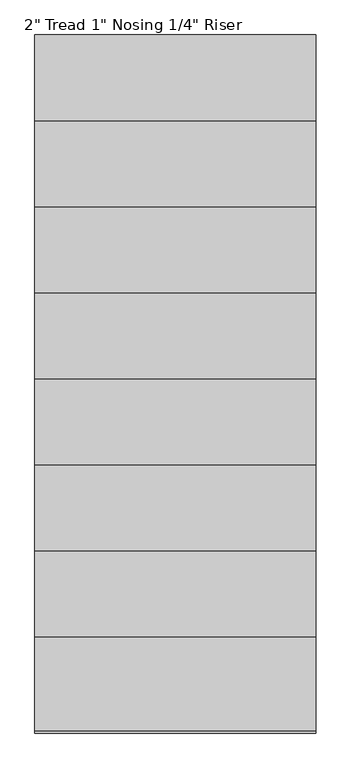
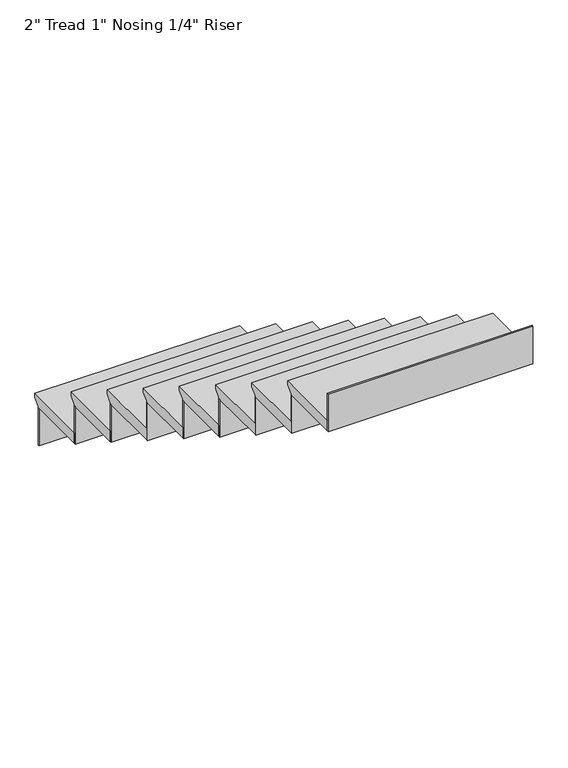
"""IFC4 building model written with IfcOpenShell, lengths in millimetres: stair flight geometry."""

from ifc_helpers import new_model, si_unit, frame, origin, place, context, project, spatial, polyline, outline, extrude, source, transform, mapped, element, save


def stair_flight_b3fe96e5(model_context):
    return source(origin(), model_context, "Body", "SweptSolid", [
        extrude(outline(polyline([(12995.2419954, 1778.0), (13300.0419954, 1778.0), (13300.0419954, 1758.95), (13274.6419954, 1733.55), (13274.6419954, 1727.2), (12995.2419954, 1727.2), (12995.2419954, 1778.0)])), frame((-5762.1737939, 0.0, 0.0), z_axis=(1.0, 0.0, 0.0), x_axis=(0.0, 1.0, 0.0)), (0.0, 0.0, 1.0), 914.4),
        extrude(outline(polyline([(-5762.1737939, 13268.2919954), (-5762.1737939, 13274.6419954), (-4847.7737939, 13274.6419954), (-4847.7737939, 13268.2919954), (-5762.1737939, 13268.2919954)])), frame((0.0, 0.0, 1549.4), z_axis=(0.0, 0.0, 1.0), x_axis=(1.0, 0.0, 0.0)), (0.0, 0.0, 1.0), 177.8),
        extrude(outline(polyline([(-5762.1737939, 12988.8919954), (-5762.1737939, 12995.2419954), (-4847.7737939, 12995.2419954), (-4847.7737939, 12988.8919954), (-5762.1737939, 12988.8919954)])), frame((0.0, 0.0, 1727.2), z_axis=(0.0, 0.0, 1.0), x_axis=(1.0, 0.0, 0.0)), (0.0, 0.0, 1.0), 177.8),
        extrude(outline(polyline([(12715.8419954, 1955.8), (13020.6419954, 1955.8), (13020.6419954, 1936.75), (12995.2419954, 1911.35), (12995.2419954, 1905.0), (12715.8419954, 1905.0), (12715.8419954, 1955.8)])), frame((-5762.1737939, 0.0, 0.0), z_axis=(1.0, 0.0, 0.0), x_axis=(0.0, 1.0, 0.0)), (0.0, 0.0, 1.0), 914.4),
        extrude(outline(polyline([(-5762.1737939, 12709.4919954), (-5762.1737939, 12715.8419954), (-4847.7737939, 12715.8419954), (-4847.7737939, 12709.4919954), (-5762.1737939, 12709.4919954)])), frame((0.0, 0.0, 1905.0), z_axis=(0.0, 0.0, 1.0), x_axis=(1.0, 0.0, 0.0)), (0.0, 0.0, 1.0), 177.8),
        extrude(outline(polyline([(12436.4419954, 2133.6), (12741.2419954, 2133.6), (12741.2419954, 2114.55), (12715.8419954, 2089.15), (12715.8419954, 2082.8), (12436.4419954, 2082.8), (12436.4419954, 2133.6)])), frame((-5762.1737939, 0.0, 0.0), z_axis=(1.0, 0.0, 0.0), x_axis=(0.0, 1.0, 0.0)), (0.0, 0.0, 1.0), 914.4),
        extrude(outline(polyline([(-5762.1737939, 12430.0919954), (-5762.1737939, 12436.4419954), (-4847.7737939, 12436.4419954), (-4847.7737939, 12430.0919954), (-5762.1737939, 12430.0919954)])), frame((0.0, 0.0, 2082.8), z_axis=(0.0, 0.0, 1.0), x_axis=(1.0, 0.0, 0.0)), (0.0, 0.0, 1.0), 177.8),
        extrude(outline(polyline([(12157.0419954, 2311.4), (12461.8419954, 2311.4), (12461.8419954, 2292.35), (12436.4419954, 2266.95), (12436.4419954, 2260.6), (12157.0419954, 2260.6), (12157.0419954, 2311.4)])), frame((-5762.1737939, 0.0, 0.0), z_axis=(1.0, 0.0, 0.0), x_axis=(0.0, 1.0, 0.0)), (0.0, 0.0, 1.0), 914.4),
        extrude(outline(polyline([(-5762.1737939, 12150.6919954), (-5762.1737939, 12157.0419954), (-4847.7737939, 12157.0419954), (-4847.7737939, 12150.6919954), (-5762.1737939, 12150.6919954)])), frame((0.0, 0.0, 2260.6), z_axis=(0.0, 0.0, 1.0), x_axis=(1.0, 0.0, 0.0)), (0.0, 0.0, 1.0), 177.8),
        extrude(outline(polyline([(11877.6419954, 2489.2), (12182.4419954, 2489.2), (12182.4419954, 2470.15), (12157.0419954, 2444.75), (12157.0419954, 2438.4), (11877.6419954, 2438.4), (11877.6419954, 2489.2)])), frame((-5762.1737939, 0.0, 0.0), z_axis=(1.0, 0.0, 0.0), x_axis=(0.0, 1.0, 0.0)), (0.0, 0.0, 1.0), 914.4),
        extrude(outline(polyline([(-5762.1737939, 11871.2919954), (-5762.1737939, 11877.6419954), (-4847.7737939, 11877.6419954), (-4847.7737939, 11871.2919954), (-5762.1737939, 11871.2919954)])), frame((0.0, 0.0, 2438.4), z_axis=(0.0, 0.0, 1.0), x_axis=(1.0, 0.0, 0.0)), (0.0, 0.0, 1.0), 177.8),
        extrude(outline(polyline([(11598.2419954, 2667.0), (11903.0419954, 2667.0), (11903.0419954, 2647.95), (11877.6419954, 2622.55), (11877.6419954, 2616.2), (11598.2419954, 2616.2), (11598.2419954, 2667.0)])), frame((-5762.1737939, 0.0, 0.0), z_axis=(1.0, 0.0, 0.0), x_axis=(0.0, 1.0, 0.0)), (0.0, 0.0, 1.0), 914.4),
        extrude(outline(polyline([(-5762.1737939, 11591.8919954), (-5762.1737939, 11598.2419954), (-4847.7737939, 11598.2419954), (-4847.7737939, 11591.8919954), (-5762.1737939, 11591.8919954)])), frame((0.0, 0.0, 2616.2), z_axis=(0.0, 0.0, 1.0), x_axis=(1.0, 0.0, 0.0)), (0.0, 0.0, 1.0), 177.8),
        extrude(outline(polyline([(11318.8419954, 2844.8), (11623.6419954, 2844.8), (11623.6419954, 2825.75), (11598.2419954, 2800.35), (11598.2419954, 2794.0), (11318.8419954, 2794.0), (11318.8419954, 2844.8)])), frame((-5762.1737939, 0.0, 0.0), z_axis=(1.0, 0.0, 0.0), x_axis=(0.0, 1.0, 0.0)), (0.0, 0.0, 1.0), 914.4),
        extrude(outline(polyline([(-5762.1737939, 11312.4919954), (-5762.1737939, 11318.8419954), (-4847.7737939, 11318.8419954), (-4847.7737939, 11312.4919954), (-5762.1737939, 11312.4919954)])), frame((0.0, 0.0, 2794.0), z_axis=(0.0, 0.0, 1.0), x_axis=(1.0, 0.0, 0.0)), (0.0, 0.0, 1.0), 177.8),
        extrude(outline(polyline([(-5762.1737939, 11033.0919954), (-5762.1737939, 11039.4419954), (-4847.7737939, 11039.4419954), (-4847.7737939, 11033.0919954), (-5762.1737939, 11033.0919954)])), frame((0.0, 0.0, 2971.8), z_axis=(0.0, 0.0, 1.0), x_axis=(1.0, 0.0, 0.0)), (0.0, 0.0, 1.0), 177.8),
        extrude(outline(polyline([(11039.4419954, 3022.6), (11344.2419954, 3022.6), (11344.2419954, 3003.55), (11318.8419954, 2978.15), (11318.8419954, 2971.8), (11039.4419954, 2971.8), (11039.4419954, 3022.6)])), frame((-5762.1737939, 0.0, 0.0), z_axis=(1.0, 0.0, 0.0), x_axis=(0.0, 1.0, 0.0)), (0.0, 0.0, 1.0), 914.4),
    ])


if __name__ == "__main__":
    model = new_model("IFC4")
    model_context = context("Model", 3, world=origin())
    ifc_project = project(units=[si_unit("LENGTHUNIT", "METRE", prefix="MILLI")], contexts=[model_context])
    site = spatial("IfcSite", under=ifc_project)
    building = spatial("IfcBuilding", under=site)
    placement = place(None, origin())
    stair_flight_shape = stair_flight_b3fe96e5(model_context)
    element("IfcStairFlight", 1, ObjectType="2\" Tread 1\" Nosing 1/4\" Riser", at=placement, inside=building, context=model_context, shape_type="MappedRepresentation", body=[
        mapped(stair_flight_shape, transform((0.0, 0.0, 0.0), x_axis=(1.0, 0.0, 0.0), y_axis=(0.0, 1.0, 0.0), z_axis=(0.0, 0.0, 1.0))),
    ])
    save(model, "model.ifc")
